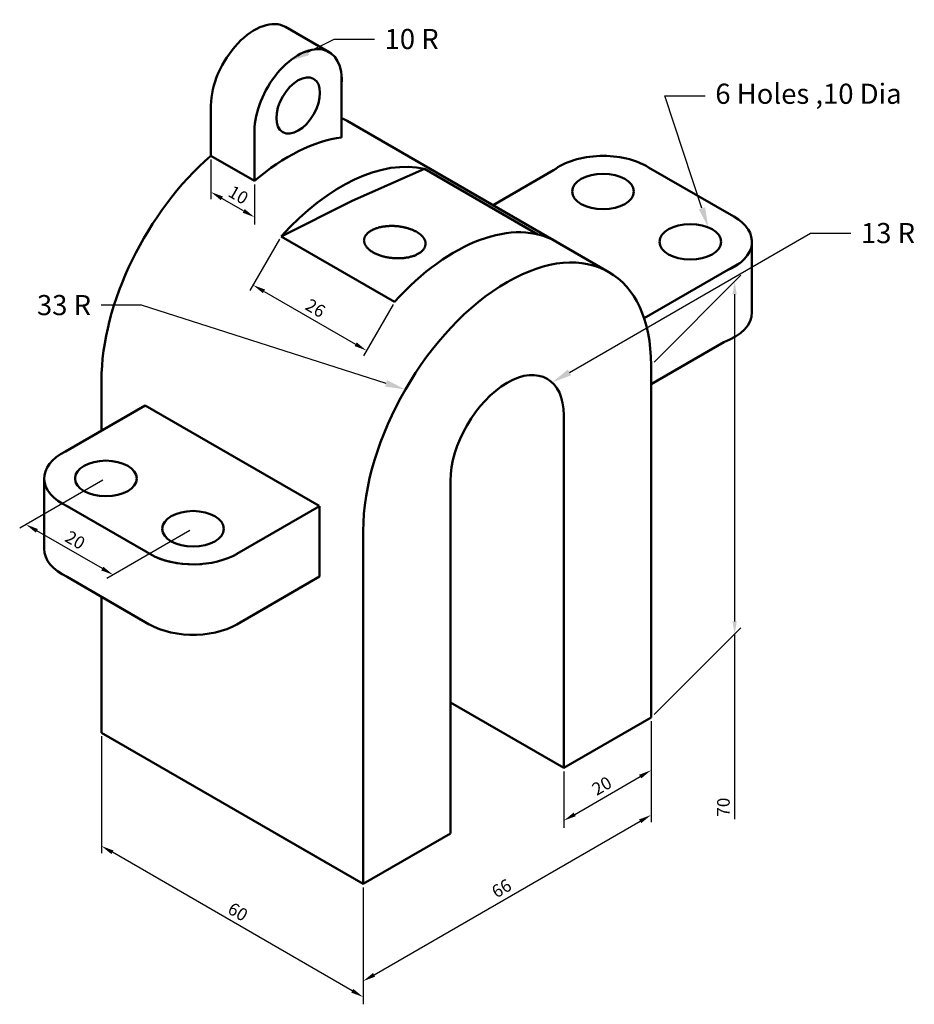
# Model space of a CAD drawing. Units: millimetres. Extents: x 4116 to 4293, y 813 to 1008.
import ezdxf
from ezdxf import colors
from ezdxf.entities.mleader import LeaderData, LeaderLine
from ezdxf.math import Vec2, Vec3

# ---------------------------------------------------------------- set-up
doc = ezdxf.new("R2010")
doc.units = ezdxf.units.MM
for name, color, linetype, lineweight in [('M-DIMS', 2, 'Continuous', 25), ('M-OUTL', 7, 'Continuous', 50), ('M-TEXT', 3, 'Continuous', 25)]:
    doc.layers.add(name, color=color, linetype=linetype, lineweight=lineweight)
doc.styles.get("Standard").update_dxf_attribs({"font": 'arial.ttf'})
doc.dimstyles.new('ISO-25', dxfattribs={"dimtxt": 2.5, "dimasz": 2.5, "dimexe": 1.25, "dimexo": 0.625, "dimtad": 1, "dimtxsty": 'Standard', "dimcen": 2.5, "dimadec": 0, "dimazin": 0, "dimtfac": 1, "dimtmove": 0, "dimatfit": 3, "dimfxl": 1, "dimarcsym": 0})

# ---------------------------------------------------------------- blocks, each defined once
blk = doc.blocks.new('*D1')
at = {"layer": 'Defpoints', "color": 0, "transparency": 16777216}
for p in [(4132.04, 866.65), (4132.04, 844.14), (4184, 836.65)]:
    blk.add_point(p, dxfattribs=at)
at = {"layer": 'M-DIMS', "color": 0, "lineweight": -2, "transparency": 16777216}
for p, q in [((4132.04, 865.93), (4132.04, 842.7)), ((4181.84, 815.39), (4134.21, 842.89)), ((4184, 835.93), (4184, 812.7))]:
    blk.add_line(p, q, dxfattribs=at)
at = {"layer": 'M-DIMS', "color": 0, "transparency": 16777216}
for points in [[(4134.42, 843.25), (4134, 842.53), (4132.04, 844.14)], [(4182.05, 815.75), (4181.63, 815.03), (4184, 814.14)]]:
    blk.add_solid(points, dxfattribs=at)
at = {"layer": 'M-DIMS', "color": 0, "transparency": 16777216, "insert": (4158.97, 830.79), "char_height": 2.5, "attachment_point": 5, "rotation": 330}
blk.add_mtext('60', dxfattribs=at)
blk = doc.blocks.new('*D2')
at = {"layer": 'Defpoints', "color": 0, "transparency": 16777216}
for p in [(4241.16, 869.65), (4241.16, 850.3), (4184, 836.65)]:
    blk.add_point(p, dxfattribs=at)
at = {"layer": 'M-DIMS', "color": 0, "lineweight": -2, "transparency": 16777216}
for p, q in [((4241.16, 868.93), (4241.16, 848.86)), ((4186.17, 818.55), (4239, 849.05)), ((4184, 835.93), (4184, 815.86))]:
    blk.add_line(p, q, dxfattribs=at)
at = {"layer": 'M-DIMS', "color": 0, "transparency": 16777216}
for points in [[(4238.79, 849.42), (4239.21, 848.69), (4241.16, 850.3)], [(4185.96, 818.92), (4186.38, 818.19), (4184, 817.3)]]:
    blk.add_solid(points, dxfattribs=at)
at = {"layer": 'M-DIMS', "color": 0, "transparency": 16777216, "insert": (4211.63, 835.45), "char_height": 2.5, "attachment_point": 5, "rotation": 30}
blk.add_mtext('66', dxfattribs=at)
blk = doc.blocks.new('*D3')
at = {"layer": 'Defpoints', "color": 0, "transparency": 16777216}
for p in [(4241.16, 869.65), (4223.84, 859.65), (4241.16, 859.18)]:
    blk.add_point(p, dxfattribs=at)
at = {"layer": 'M-DIMS', "color": 0, "lineweight": -2, "transparency": 16777216}
for p, q in [((4241.16, 868.93), (4241.16, 857.73)), ((4223.84, 858.93), (4223.84, 847.73)), ((4226.01, 850.43), (4239, 857.93))]:
    blk.add_line(p, q, dxfattribs=at)
at = {"layer": 'M-DIMS', "color": 0, "transparency": 16777216}
for points in [[(4238.79, 858.29), (4239.21, 857.57), (4241.16, 859.18)], [(4225.8, 850.79), (4226.21, 850.07), (4223.84, 849.18)]]:
    blk.add_solid(points, dxfattribs=at)
at = {"layer": 'M-DIMS', "color": 0, "transparency": 16777216, "insert": (4231.55, 855.82), "char_height": 2.5, "attachment_point": 5, "rotation": 30}
blk.add_mtext('20', dxfattribs=at)
blk = doc.blocks.new('*D4')
at = {"layer": 'Defpoints', "color": 0, "transparency": 16777216}
for p in [(4257.76, 956.25), (4241.16, 939.65), (4241.16, 869.65)]:
    blk.add_point(p, dxfattribs=at)
at = {"layer": 'M-DIMS', "color": 0, "lineweight": -2, "transparency": 16777216}
for p, q in [((4241.79, 940.28), (4259.01, 957.51)), ((4257.76, 953.75), (4257.76, 888.75)), ((4241.79, 870.28), (4259.01, 887.51)), ((4257.76, 886.25), (4257.76, 849.45))]:
    blk.add_line(p, q, dxfattribs=at)
at = {"layer": 'M-DIMS', "color": 0, "transparency": 16777216}
for points in [[(4257.34, 953.75), (4258.18, 953.75), (4257.76, 956.25)], [(4257.34, 888.75), (4258.18, 888.75), (4257.76, 886.25)]]:
    blk.add_solid(points, dxfattribs=at)
at = {"layer": 'M-DIMS', "color": 0, "transparency": 16777216, "insert": (4255.86, 851.85), "char_height": 2.5, "attachment_point": 5, "rotation": 90}
blk.add_mtext('70', dxfattribs=at)
blk = doc.blocks.new('*D5')
at = {"layer": 'Defpoints', "color": 0, "transparency": 16777216}
for p in [(4167.73, 965.24), (4190.25, 952.24), (4184.66, 942.56)]:
    blk.add_point(p, dxfattribs=at)
at = {"layer": 'M-DIMS', "color": 0, "lineweight": -2, "transparency": 16777216}
for p, q in [((4167.42, 964.7), (4161.52, 954.48)), ((4164.31, 954.31), (4182.5, 943.81)), ((4189.94, 951.7), (4184.04, 941.48))]:
    blk.add_line(p, q, dxfattribs=at)
at = {"layer": 'M-DIMS', "color": 0, "transparency": 16777216}
for points in [[(4164.52, 954.67), (4164.1, 953.95), (4162.15, 955.56)], [(4182.71, 944.17), (4182.29, 943.45), (4184.66, 942.56)]]:
    blk.add_solid(points, dxfattribs=at)
at = {"layer": 'M-DIMS', "color": 0, "transparency": 16777216, "insert": (4174.36, 950.71), "char_height": 2.5, "attachment_point": 5, "rotation": 330}
blk.add_mtext('26', dxfattribs=at)
blk = doc.blocks.new('*D6')
at = {"layer": 'Defpoints', "color": 0, "transparency": 16777216}
for p in [(4153.78, 981.24), (4162.44, 976.24), (4153.78, 974.04)]:
    blk.add_point(p, dxfattribs=at)
at = {"layer": 'M-DIMS', "color": 0, "lineweight": -2, "transparency": 16777216}
for p, q in [((4153.78, 980.52), (4153.78, 972.6)), ((4162.44, 975.52), (4162.44, 967.6)), ((4160.27, 970.29), (4155.94, 972.79))]:
    blk.add_line(p, q, dxfattribs=at)
at = {"layer": 'M-DIMS', "color": 0, "transparency": 16777216}
for points in [[(4156.15, 973.15), (4155.73, 972.43), (4153.78, 974.04)], [(4160.48, 970.65), (4160.06, 969.93), (4162.44, 969.04)]]:
    blk.add_solid(points, dxfattribs=at)
at = {"layer": 'M-DIMS', "color": 0, "transparency": 16777216, "insert": (4159.06, 973.19), "char_height": 2.5, "attachment_point": 5, "rotation": 330}
blk.add_mtext('10', dxfattribs=at)
blk = doc.blocks.new('*D7')
at = {"layer": 'Defpoints', "color": 0, "transparency": 16777216}
for p in [(4132.91, 917.15), (4117.05, 908), (4150.23, 907.15)]:
    blk.add_point(p, dxfattribs=at)
at = {"layer": 'M-DIMS', "color": 0, "lineweight": -2, "transparency": 16777216}
for p, q in [((4132.28, 916.79), (4115.8, 907.27)), ((4132.21, 899.25), (4119.22, 906.75)), ((4149.6, 906.79), (4133.12, 897.27))]:
    blk.add_line(p, q, dxfattribs=at)
at = {"layer": 'M-DIMS', "color": 0, "transparency": 16777216}
for points in [[(4119.42, 907.11), (4119.01, 906.38), (4117.05, 908)], [(4132.41, 899.61), (4132, 898.88), (4134.37, 898)]]:
    blk.add_solid(points, dxfattribs=at)
at = {"layer": 'M-DIMS', "color": 0, "transparency": 16777216, "insert": (4126.66, 904.64), "char_height": 2.5, "attachment_point": 5, "rotation": 330}
blk.add_mtext('20', dxfattribs=at)

msp = doc.modelspace()

# ---------------------------------------------------------------- linework, layer by layer
at = {"layer": 'M-OUTL'}
for p, q in [((4168.559, 1006.844), (4177.219, 1001.844)), ((4179.714, 997.196), (4179.714, 984.897)), ((4153.775, 981.237), (4153.775, 991.237)), ((4180.83, 988.153), (4232.791, 958.153)), ((4162.436, 981.237), (4162.436, 986.237)), ((4153.775, 981.237), (4162.436, 976.237)), ((4162.436, 976.237), (4162.436, 981.237)), ((4181.848, 972.31), (4196.176, 978.621)), ((4196.176, 978.621), (4218.693, 965.621)), ((4221.805, 978.368), (4209.791, 971.432)), ((4240.647, 978.939), (4257.612, 969.153)), ((4167.734, 965.24), (4181.848, 972.31)), ((4167.734, 965.24), (4190.251, 952.24)), ((4261.203, 964.151), (4261.203, 950.151)), ((4258.743, 959.9), (4239.791, 948.958)), ((4255.583, 944.204), (4241.162, 935.878)), ((4241.162, 869.651), (4241.162, 939.651)), ((4132.043, 926.626), (4132.043, 936.651)), ((4124.885, 922.493), (4140.725, 931.638)), ((4140.725, 931.638), (4175.291, 911.681)), ((4223.841, 929.651), (4223.841, 859.651)), ((4120.661, 917.151), (4120.661, 903.151)), ((4201.325, 916.651), (4201.325, 846.651)), ((4125.251, 911.632), (4142.572, 901.632)), ((4175.343, 911.651), (4158.889, 902.151)), ((4175.343, 897.651), (4175.343, 911.651)), ((4184.004, 836.651), (4184.004, 906.651)), ((4125.251, 897.632), (4141.541, 888.167)), ((4175.343, 897.651), (4158.889, 888.151)), ((4132.043, 866.651), (4132.043, 893.686)), ((4223.841, 859.651), (4201.325, 872.651)), ((4223.841, 859.651), (4241.162, 869.651)), ((4184.004, 836.651), (4132.043, 866.651)), ((4184.004, 836.651), (4166.684, 846.651)), ((4184.004, 836.651), (4201.325, 846.651))]:
    msp.add_line(p, q, dxfattribs=at)
for points in [[(4184.158, 964.409), (4184.171, 964.487), (4184.184, 964.565), (4184.196, 964.642), (4184.209, 964.72), (4184.221, 964.798), (4184.234, 964.876), (4184.25, 964.953), (4184.288, 965.027), (4184.325, 965.102), (4184.363, 965.176), (4184.4, 965.25), (4184.438, 965.324), (4184.475, 965.399), (4184.52, 965.471), (4184.581, 965.54), (4184.642, 965.608), (4184.703, 965.677), (4184.765, 965.746), (4184.826, 965.814), (4184.887, 965.883), (4184.958, 965.948), (4185.042, 966.009), (4185.125, 966.07), (4185.208, 966.131), (4185.292, 966.193), (4185.375, 966.254), (4185.459, 966.315), (4185.553, 966.37), (4185.656, 966.422), (4185.76, 966.474), (4185.863, 966.526), (4185.966, 966.577), (4186.069, 966.629), (4186.172, 966.681), (4186.287, 966.725), (4186.407, 966.766), (4186.527, 966.807), (4186.647, 966.848), (4186.767, 966.889), (4186.887, 966.93), (4187.007, 966.971), (4187.138, 967.002), (4187.272, 967.031), (4187.405, 967.06), (4187.539, 967.089), (4187.672, 967.118), (4187.805, 967.147), (4187.939, 967.176), (4188.082, 967.193), (4188.225, 967.209), (4188.368, 967.225), (4188.511, 967.242), (4188.654, 967.258), (4188.797, 967.274), (4188.941, 967.289), (4189.089, 967.292), (4189.238, 967.295), (4189.387, 967.298), (4189.535, 967.301), (4189.684, 967.305), (4189.833, 967.308), (4189.982, 967.307), (4190.132, 967.297), (4190.282, 967.287), (4190.432, 967.277), (4190.582, 967.266), (4190.732, 967.256), (4190.882, 967.246), (4191.031, 967.23), (4191.178, 967.207), (4191.325, 967.184), (4191.473, 967.161), (4191.62, 967.138), (4191.767, 967.115), (4191.914, 967.092), (4192.058, 967.061), (4192.198, 967.026), (4192.338, 966.99), (4192.478, 966.955), (4192.619, 966.919), (4192.759, 966.884), (4192.899, 966.848), (4193.031, 966.805), (4193.161, 966.758), (4193.29, 966.711), (4193.419, 966.664), (4193.549, 966.617), (4193.678, 966.571), (4193.807, 966.524), (4193.924, 966.468), (4194.039, 966.411), (4194.153, 966.355), (4194.268, 966.298), (4194.383, 966.241), (4194.498, 966.184), (4194.612, 966.127)], [(4196.406, 963.761), (4196.383, 963.658), (4196.361, 963.555), (4196.339, 963.452), (4196.316, 963.349), (4196.294, 963.246), (4196.271, 963.143), (4196.243, 963.041), (4196.177, 962.946), (4196.111, 962.85), (4196.045, 962.755), (4195.979, 962.659), (4195.913, 962.564), (4195.847, 962.468), (4195.769, 962.376), (4195.663, 962.293), (4195.556, 962.21), (4195.45, 962.127), (4195.343, 962.043), (4195.237, 961.96), (4195.131, 961.877), (4195.009, 961.801), (4194.868, 961.734), (4194.726, 961.668), (4194.585, 961.601), (4194.444, 961.534), (4194.302, 961.468), (4194.161, 961.401), (4194.003, 961.345), (4193.834, 961.299), (4193.665, 961.252), (4193.495, 961.205), (4193.326, 961.158), (4193.157, 961.111), (4192.987, 961.064), (4192.804, 961.033), (4192.616, 961.009), (4192.427, 960.984), (4192.238, 960.959), (4192.049, 960.935), (4191.86, 960.91), (4191.672, 960.885), (4191.474, 960.881), (4191.276, 960.88), (4191.077, 960.878), (4190.878, 960.877), (4190.68, 960.876), (4190.481, 960.875), (4190.282, 960.873), (4190.083, 960.896), (4189.885, 960.918), (4189.686, 960.94), (4189.487, 960.962), (4189.288, 960.985), (4189.09, 961.007), (4188.892, 961.032), (4188.704, 961.077), (4188.515, 961.122), (4188.326, 961.166), (4188.137, 961.211), (4187.949, 961.256), (4187.76, 961.3), (4187.577, 961.351), (4187.407, 961.415), (4187.238, 961.48), (4187.069, 961.545), (4186.899, 961.61), (4186.73, 961.674), (4186.561, 961.739), (4186.403, 961.811), (4186.262, 961.893), (4186.121, 961.974), (4185.979, 962.056), (4185.838, 962.138), (4185.696, 962.219), (4185.555, 962.301), (4185.434, 962.39), (4185.327, 962.484), (4185.221, 962.579), (4185.114, 962.673), (4185.008, 962.768), (4184.902, 962.862), (4184.795, 962.956), (4184.718, 963.057), (4184.652, 963.159), (4184.586, 963.262), (4184.519, 963.364), (4184.453, 963.467), (4184.387, 963.569), (4184.321, 963.672), (4184.293, 963.777), (4184.27, 963.882), (4184.248, 963.987), (4184.226, 964.093), (4184.203, 964.198), (4184.181, 964.304), (4184.158, 964.409)], [(4194.612, 966.127), (4194.647, 966.106), (4194.681, 966.085), (4194.715, 966.064), (4194.75, 966.044), (4194.784, 966.023), (4194.819, 966.002), (4194.853, 965.981), (4194.885, 965.959), (4194.917, 965.937), (4194.95, 965.915), (4194.982, 965.894), (4195.014, 965.872), (4195.047, 965.85), (4195.078, 965.828), (4195.109, 965.805), (4195.139, 965.783), (4195.169, 965.76), (4195.199, 965.738), (4195.229, 965.715), (4195.259, 965.692), (4195.288, 965.67), (4195.316, 965.646), (4195.344, 965.623), (4195.372, 965.6), (4195.4, 965.576), (4195.427, 965.553), (4195.455, 965.53), (4195.482, 965.506), (4195.507, 965.482), (4195.533, 965.458), (4195.558, 965.434), (4195.584, 965.41), (4195.609, 965.386), (4195.634, 965.362), (4195.658, 965.338), (4195.681, 965.313), (4195.704, 965.289), (4195.727, 965.264), (4195.75, 965.239), (4195.773, 965.215), (4195.796, 965.19), (4195.817, 965.165), (4195.837, 965.14), (4195.858, 965.115), (4195.878, 965.09), (4195.899, 965.065), (4195.919, 965.04), (4195.94, 965.015), (4195.958, 964.99), (4195.975, 964.964), (4195.993, 964.939), (4196.011, 964.913), (4196.029, 964.888), (4196.047, 964.862), (4196.064, 964.837), (4196.08, 964.811), (4196.095, 964.785), (4196.11, 964.759), (4196.125, 964.733), (4196.14, 964.707), (4196.156, 964.682), (4196.17, 964.656), (4196.183, 964.629), (4196.195, 964.603), (4196.208, 964.577), (4196.22, 964.551), (4196.233, 964.525), (4196.245, 964.499), (4196.256, 964.473), (4196.266, 964.447), (4196.276, 964.42), (4196.286, 964.394), (4196.296, 964.368), (4196.305, 964.341), (4196.315, 964.315), (4196.323, 964.289), (4196.33, 964.262), (4196.337, 964.236), (4196.344, 964.21), (4196.351, 964.183), (4196.358, 964.157), (4196.365, 964.13), (4196.37, 964.104), (4196.375, 964.078), (4196.379, 964.051), (4196.383, 964.025), (4196.387, 963.998), (4196.391, 963.972), (4196.396, 963.946), (4196.397, 963.919), (4196.399, 963.893), (4196.4, 963.867), (4196.402, 963.84), (4196.403, 963.814), (4196.404, 963.788), (4196.406, 963.761)]]:
    msp.add_lwpolyline(points, dxfattribs=at)
for centre, major_axis, start_param, end_param in [((4162.436, 996.237), (-6.124, -10.607), 3.1415927, 5.4977871), ((4171.096, 991.237), (-6.124, -10.607), 2.2577837, 5.4977871), ((4160.621, 953.151), (-20.208, -35.002), 3.1415927, 3.1953749), ((4169.282, 948.151), (-20.208, -35.002), 3.5533123, 4.168895), ((4160.621, 953.151), (-20.208, -35.002), 4.168895, 5.4977871), ((4179.674, 942.151), (-20.208, -35.002), 3.3114124, 4.3579938), ((4231.635, 974.151), (-12.247, 0), 3.8855316, 5.6441168), ((4202.191, 929.151), (-20.208, -35.002), 3.1415927, 4.3579938), ((4248.956, 964.151), (-12.247, 0), 2.2157693, 3.9274296), ((4212.583, 923.151), (-20.208, -35.002), 2.3561945, 5.4977871), ((4240.296, 959.151), (-12.247, 0), 1.4174494, 1.4288993), ((4240.296, 945.151), (-12.247, 0), 11.1374713, 11.1479173), ((4248.956, 950.151), (-12.247, 0), 8.4257096, 9.424778), ((4212.583, 923.151), (-7.961, -13.789), 2.3561945, 5.4977871), ((4132.909, 917.151), (-12.247, 0), 5.4267001, 7.1785779), ((4132.909, 903.151), (-12.247, 0), 6.2831853, 7.1785779), ((4150.229, 907.151), (-12.247, 0), 7.1785779, 8.7496752), ((4150.229, 907.151), (-12.247, 0), 0.8953925, 1.7126934), ((4150.229, 893.151), (-12.247, 0), 7.0653837, 8.7496752)]:
    msp.add_ellipse(centre, major_axis=major_axis, ratio=0.5773503, start_param=start_param, end_param=end_param, dxfattribs=at)
for centre, major_axis in [((4171.096, 991.237), (-3.062, -5.303)), ((4231.635, 974.151), (-6.124, 0)), ((4231.635, 974.151), (-6.124, 0)), ((4248.956, 964.151), (-6.124, 0)), ((4248.956, 964.151), (-6.124, 0)), ((4132.909, 917.151), (-6.124, 0)), ((4150.229, 907.151), (-6.124, 0))]:
    msp.add_ellipse(centre, major_axis=major_axis, ratio=0.5773503, dxfattribs=at)

# ---------------------------------------------------------------- dimensions: what is measured, and where the dimension line sits
at = {"layer": 'M-DIMS'}
for p1, p2, distance, picture, middle in [((4162.436, 976.237), (4153.775, 981.237), 6.233, '*D6', (4159.056, 973.187)), ((4167.734, 965.24), (4190.251, 952.24), -11.174, '*D5', (4174.356, 950.709)), ((4150.229, 907.151), (4132.909, 917.151), 15.858, '*D7', (4126.662, 904.642)), ((4184.004, 836.651), (4241.162, 869.651), -16.754, '*D2', (4211.632, 835.451)), ((4223.841, 859.651), (4241.162, 869.651), -9.071, '*D3', (4231.551, 855.823)), ((4184.004, 836.651), (4132.043, 866.651), 19.494, '*D1', (4158.974, 830.788))]:
    dim = msp.add_aligned_dim(p1=p1, p2=p2, distance=distance, dimstyle='ISO-25', override={"dimclrd": 0, "dimclre": 0, "dimclrt": 0}, dxfattribs=at)
    dim.commit()
    dim.dimension.update_dxf_attribs({"geometry": picture, "text_midpoint": middle})
dim = msp.add_linear_dim(base=(4257.76, 956.255), p1=(4241.162, 869.651), p2=(4241.162, 939.651), angle=90, dimstyle='ISO-25', override={"dimclrd": 0, "dimclre": 0, "dimclrt": 0}, dxfattribs=at)
dim.commit()
dim.dimension.update_dxf_attribs({"geometry": '*D4', "text_midpoint": (4257.76, 851.846), "dimtype": 161})

# ---------------------------------------------------------------- leaders
at = {"layer": 'M-TEXT'}
ml = msp.add_multileader_mtext('Standard', dxfattribs=at)
ml.set_content('10 R ', color=256)
ml.set_leader_properties()
ml.build(insert=Vec2(0, 0))
ctx = ml.context
ctx.base_point, ctx.plane_origin = Vec3(4186.251, 1004.404), Vec3(4169.408, 1000.071)
notes = []
notes.append((ctx, [(0, (1, 1, 0), (4178.251, 1004.404), (1, 0), 8, [(0, [(4169.408, 1000.071)], 0, [])])]))
ctx.mtext.insert, ctx.mtext.flow_direction = Vec3(4188.251, 1006.438), 5
ml = msp.add_multileader_mtext('Standard', dxfattribs=at)
ml.set_content('6 Holes ,10 Dia', color=256)
ml.set_leader_properties()
ml.build(insert=Vec2(0, 0))
ctx = ml.context
ctx.base_point, ctx.plane_origin = Vec3(4251.918, 993.166), Vec3(4252.527, 967.023)
notes.append((ctx, [(0, (1, 1, 0), (4243.918, 993.166), (1, 0), 8, [(0, [(4252.527, 967.023)], 0, [])])]))
ctx.mtext.insert, ctx.mtext.flow_direction = Vec3(4253.918, 995.562), 5
ml = msp.add_multileader_mtext('Standard', dxfattribs=at)
ml.set_content('13 R', color=256)
ml.set_leader_properties()
ml.build(insert=Vec2(0, 0))
ctx = ml.context
ctx.base_point, ctx.plane_origin = Vec3(4280.843, 965.854), Vec3(4221.516, 936.22)
notes.append((ctx, [(0, (1, 1, 0), (4272.843, 965.854), (1, 0), 8, [(0, [(4221.516, 936.22)], 0, [])])]))
ctx.mtext.insert, ctx.mtext.flow_direction = Vec3(4282.843, 967.889), 5
ml = msp.add_multileader_mtext('Standard', dxfattribs=at)
ml.set_content('33 R', color=256)
ml.set_leader_properties()
ml.build(insert=Vec2(0, 0))
ctx = ml.context
ctx.base_point, ctx.plane_origin = Vec3(4116.467, 951.55), Vec3(4192.375, 934.818)
ctx.text_align_type = 2
notes.append((ctx, [(0, (1, 1, 0), (4139.965, 951.55), (-1, 0), 8, [(0, [(4192.375, 934.818)], 0, [])])]))
ctx.mtext.insert, ctx.mtext.alignment, ctx.mtext.flow_direction = Vec3(4129.965, 953.585), 3, 5
for ctx, leaders in notes:
    for number, flags, end, landing, length, lines in leaders:
        leader = LeaderData()
        leader.index, (leader.has_last_leader_line, leader.has_dogleg_vector, leader.attachment_direction) = number, flags
        leader.last_leader_point, leader.dogleg_vector, leader.dogleg_length = Vec3(end), Vec3(landing), length
        for number, points, colour, breaks in lines:
            line = LeaderLine()
            line.index, line.vertices, line.color, line.breaks = number, Vec3.list(points), colors.encode_raw_color(colour), breaks
            leader.lines.append(line)
        ctx.leaders.append(leader)

doc.saveas('drawing.dxf')
